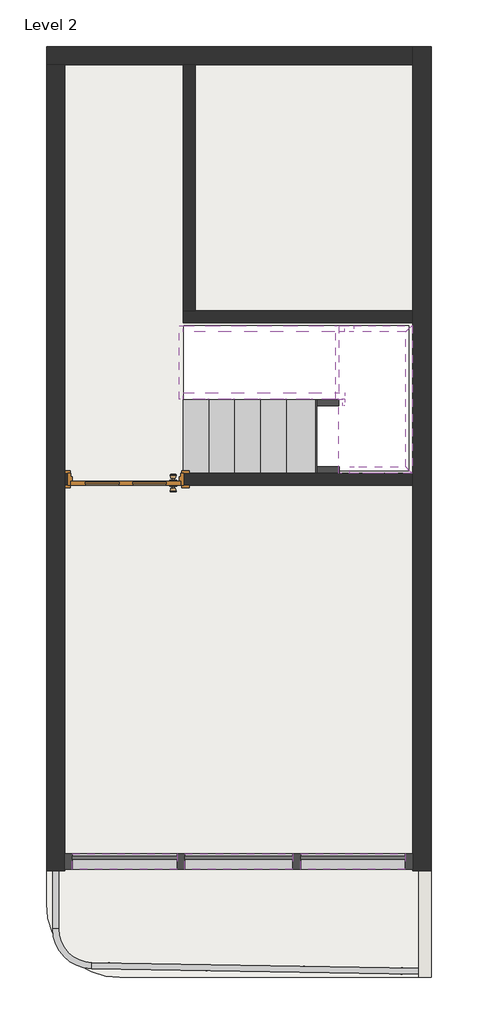
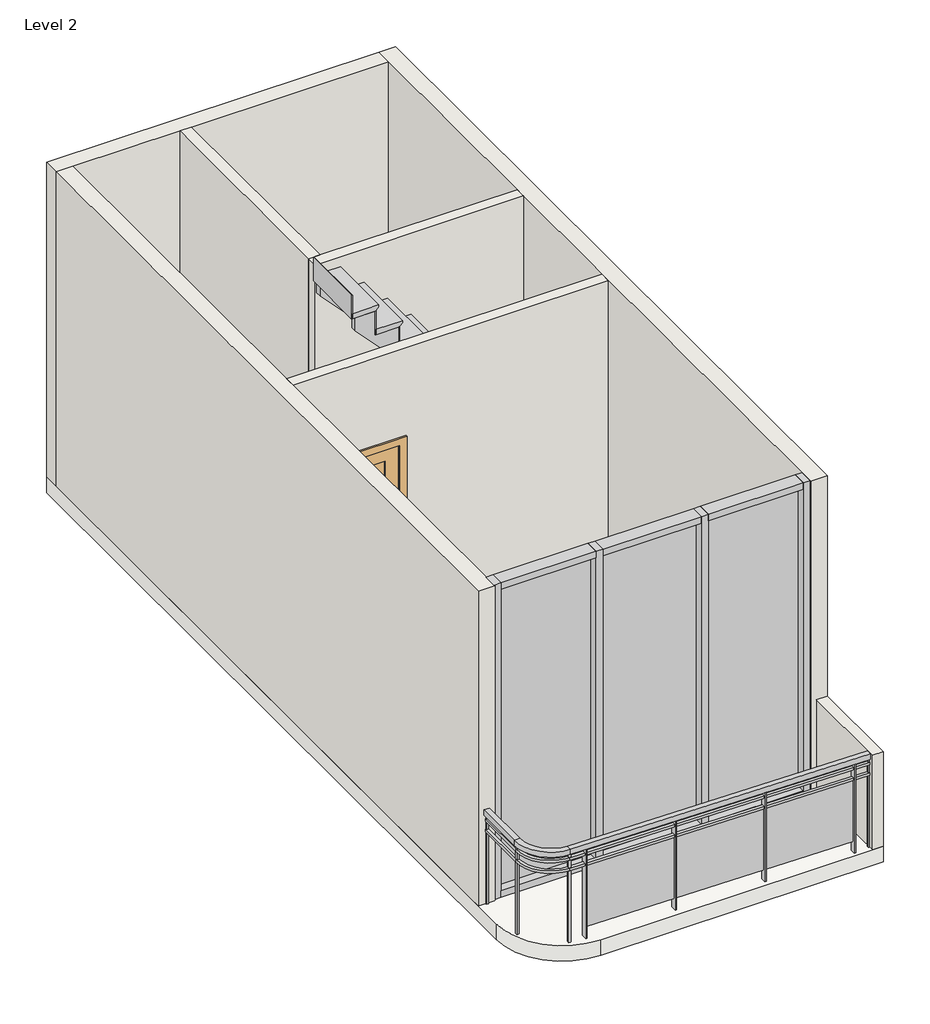
# One storey: 18 members, 7 walls, 3 plates, 2 slabs, 2 stair flights, 1 door, 1 railing.
"""IFC4 building model written with IfcOpenShell, lengths in millimetres."""

from ifc_helpers import new_model, si_unit, point, frame, frame_2d, origin, place, context, project, spatial, polyline, circle_curve, trimmed, segment, composite_curve, outline, extrude, faceted_brep, transform, mapped, element, save
from ifc_brep_helpers import plane_surface, cylinder_surface, revolved_surface, advanced_brep
from components import door_interior_single_4_panel_wood_3_aef61117, member_024c663a, member_b7368e82, member_eaba9652, member_3f395ae9, system_panel_glazed_640eda3d, system_panel_glazed_15df7e53, non_monolithic_landing_067df1a0, stair_flight_7576936b, stair_flight_48b2ccee

model = new_model("IFC4")

# Units and contexts
model_context = context("Model", 3, world=origin())
ifc_project = project(units=[si_unit("LENGTHUNIT", "METRE", prefix="MILLI")], contexts=[model_context])

# Site, building, storey
site = spatial("IfcSite", under=ifc_project)
building = spatial("IfcBuilding", under=site)
storey = spatial("IfcBuildingStorey", under=building, Name="Level 2", Elevation=3200.4)

# Door
placement = place(None, origin())
door_interior_single_4_panel_wood_3_shape = door_interior_single_4_panel_wood_3_aef61117(model_context)
element("IfcDoor", 1, ObjectType="Door-Interior-Single-4_Panel-Wood : 3'", at=placement, inside=storey, context=model_context, shape_type="MappedRepresentation", body=[
    mapped(door_interior_single_4_panel_wood_3_shape, transform((-5067.456559, 3670.9730625, 3200.4), x_axis=(-1.0, 0.0, 0.0), y_axis=(0.0, -1.0, 0.0), z_axis=(0.0, 0.0, 1.0))),
])

# Members
element("IfcMember", 2, ObjectType="Carriage - 2\" Width", at=placement, inside=storey, context=model_context, shape_type="Brep", body=[
    faceted_brep([(-3327.7737097, 4341.1083475, 4978.4), (-3327.7737097, 4391.9083475, 4978.4), (-3543.6737097, 4391.9083475, 4978.4), (-3543.6737097, 4341.1083475, 4978.4), (-3327.7737097, 4341.1083475, 4749.8), (-3327.7737097, 4391.9083475, 4749.8), (-3543.6737097, 4341.1083475, 5207.0), (-3543.6737097, 4391.9083475, 5207.0), (-3759.5737097, 4391.9083475, 5207.0), (-3759.5737097, 4341.1083475, 5207.0), (-3759.5737097, 4341.1083475, 5435.6), (-3759.5737097, 4391.9083475, 5435.6), (-3975.4737097, 4391.9083475, 5435.6), (-3975.4737097, 4341.1083475, 5435.6), (-3975.4737097, 4341.1083475, 5664.2), (-3975.4737097, 4391.9083475, 5664.2), (-4191.3737097, 4391.9083475, 5664.2), (-4191.3737097, 4341.1083475, 5664.2), (-4191.3737097, 4341.1083475, 5892.8), (-4191.3737097, 4391.9083475, 5892.8), (-4407.2737097, 4391.9083475, 5892.8), (-4407.2737097, 4341.1083475, 5892.8), (-4407.2737097, 4341.1083475, 6121.4), (-4407.2737097, 4391.9083475, 6121.4), (-4591.4237097, 4391.9083475, 6121.4), (-4591.4237097, 4341.1083475, 6121.4), (-3245.2237097, 4341.1083475, 4572.0), (-3245.2237097, 4391.9083475, 4572.0), (-3245.2237097, 4391.9083475, 4749.8), (-3245.2237097, 4341.1083475, 4749.8), (-3247.1951617, 4341.1083475, 4572.0), (-3247.1951617, 4391.9083475, 4572.0), (-4591.4237097, 4391.9083475, 5995.3008155), (-4591.4237097, 4341.1083475, 5995.3008155), (-3296.0237097, 4341.1083475, 4623.7008155), (-3327.7737097, 4341.1083475, 4657.3184625), (-3543.6737097, 4341.1083475, 4885.9184625), (-3759.5737097, 4341.1083475, 5114.5184625), (-3975.4737097, 4341.1083475, 5343.1184625), (-4191.3737097, 4341.1083475, 5571.7184625), (-4407.2737097, 4341.1083475, 5800.3184625), (-3296.0237097, 4341.1083475, 4749.8)], [[[0, 1, 2, 3]], [[1, 0, 4, 5]], [[6, 7, 8, 9]], [[3, 2, 7, 6]], [[10, 11, 12, 13]], [[9, 8, 11, 10]], [[14, 15, 16, 17]], [[13, 12, 15, 14]], [[18, 19, 20, 21]], [[17, 16, 19, 18]], [[22, 23, 24, 25]], [[21, 20, 23, 22]], [[26, 27, 28, 29]], [[26, 30, 31, 27]], [[32, 33, 25, 24]], [[31, 32, 24, 23, 20, 19, 16, 15, 12, 11, 8, 7, 2, 1, 5, 28, 27]], [[33, 32, 31, 30, 34, 35, 36, 37, 38, 39, 40]], [[30, 26, 29, 41, 4, 0, 3, 6, 9, 10, 13, 14, 17, 18, 21, 22, 25, 33, 40, 39, 38, 37, 36, 35, 34]], [[5, 4, 41, 29, 28]]]),
])
element("IfcMember", 3, ObjectType="Carriage - 2\" Width", at=placement, inside=storey, context=model_context, shape_type="Brep", body=[
    faceted_brep([(-4591.4237097, 4950.7083475, 5995.3008155), (-4591.4237097, 4899.9083475, 5995.3008155), (-4591.4237097, 4899.9083475, 6121.4), (-4591.4237097, 4950.7083475, 6121.4), (-3247.1951617, 4899.9083475, 4572.0), (-3170.555096, 4899.9083475, 4749.8), (-3327.7737097, 4899.9083475, 4749.8), (-3327.7737097, 4899.9083475, 4978.4), (-3543.6737097, 4899.9083475, 4978.4), (-3543.6737097, 4899.9083475, 5207.0), (-3759.5737097, 4899.9083475, 5207.0), (-3759.5737097, 4899.9083475, 5435.6), (-3975.4737097, 4899.9083475, 5435.6), (-3975.4737097, 4899.9083475, 5664.2), (-4191.3737097, 4899.9083475, 5664.2), (-4191.3737097, 4899.9083475, 5892.8), (-4407.2737097, 4899.9083475, 5892.8), (-4407.2737097, 4899.9083475, 6121.4), (-4407.2737097, 4950.7083475, 5800.3184625), (-4191.3737097, 4950.7083475, 5571.7184625), (-3975.4737097, 4950.7083475, 5343.1184625), (-3759.5737097, 4950.7083475, 5114.5184625), (-3543.6737097, 4950.7083475, 4885.9184625), (-3327.7737097, 4950.7083475, 4657.3184625), (-3296.0237097, 4950.7083475, 4623.7008155), (-3247.1951617, 4950.7083475, 4572.0), (-4407.2737097, 4950.7083475, 6121.4), (-4407.2737097, 4950.7083475, 5892.8), (-4191.3737097, 4950.7083475, 5892.8), (-4191.3737097, 4950.7083475, 5664.2), (-3975.4737097, 4950.7083475, 5664.2), (-3975.4737097, 4950.7083475, 5435.6), (-3759.5737097, 4950.7083475, 5435.6), (-3759.5737097, 4950.7083475, 5207.0), (-3543.6737097, 4950.7083475, 5207.0), (-3543.6737097, 4950.7083475, 4978.4), (-3327.7737097, 4950.7083475, 4978.4), (-3327.7737097, 4950.7083475, 4749.8), (-3296.0237097, 4950.7083475, 4749.8), (-3170.555096, 4950.7083475, 4749.8)], [[[0, 1, 2, 3]], [[1, 4, 5, 6, 7, 8, 9, 10, 11, 12, 13, 14, 15, 16, 17, 2]], [[1, 0, 18, 19, 20, 21, 22, 23, 24, 25, 4]], [[0, 3, 26, 27, 28, 29, 30, 31, 32, 33, 34, 35, 36, 37, 38, 39, 25, 24, 23, 22, 21, 20, 19, 18]], [[7, 36, 35, 8]], [[36, 7, 6, 37]], [[9, 34, 33, 10]], [[8, 35, 34, 9]], [[11, 32, 31, 12]], [[10, 33, 32, 11]], [[13, 30, 29, 14]], [[12, 31, 30, 13]], [[15, 28, 27, 16]], [[14, 29, 28, 15]], [[17, 26, 3, 2]], [[16, 27, 26, 17]], [[4, 25, 39, 5]], [[37, 6, 5, 39, 38]]]),
])
element("IfcMember", 4, ObjectType="Carriage - 2\" Width", at=placement, inside=storey, context=model_context, shape_type="Brep", body=[
    faceted_brep([(-4559.6737097, 4334.5480625, 3200.4), (-4424.3522576, 4334.5480625, 3200.4), (-4424.3522576, 4283.7480625, 3200.4), (-4559.6737097, 4283.7480625, 3200.4), (-3296.0237097, 4334.5480625, 4395.1008155), (-3296.0237097, 4283.7480625, 4395.1008155), (-4343.7737097, 4334.5480625, 3285.7184625), (-4127.8737097, 4334.5480625, 3514.3184625), (-3911.9737097, 4334.5480625, 3742.9184625), (-3696.0737097, 4334.5480625, 3971.5184625), (-3480.1737097, 4334.5480625, 4200.1184625), (-3296.0237097, 4334.5480625, 4521.2), (-4559.6737097, 4334.5480625, 3378.2), (-4343.7737097, 4334.5480625, 3378.2), (-4343.7737097, 4334.5480625, 3606.8), (-4127.8737097, 4334.5480625, 3606.8), (-4127.8737097, 4334.5480625, 3835.4), (-3911.9737097, 4334.5480625, 3835.4), (-3911.9737097, 4334.5480625, 4064.0), (-3696.0737097, 4334.5480625, 4064.0), (-3696.0737097, 4334.5480625, 4292.6), (-3480.1737097, 4334.5480625, 4292.6), (-3480.1737097, 4334.5480625, 4521.2), (-3480.1737097, 4283.7480625, 4521.2), (-3296.0237097, 4283.7480625, 4521.2), (-3480.1737097, 4283.7480625, 4292.6), (-3696.0737097, 4283.7480625, 4292.6), (-3696.0737097, 4283.7480625, 4064.0), (-3911.9737097, 4283.7480625, 4064.0), (-3911.9737097, 4283.7480625, 3835.4), (-4127.8737097, 4283.7480625, 3835.4), (-4127.8737097, 4283.7480625, 3606.8), (-4343.7737097, 4283.7480625, 3606.8), (-4343.7737097, 4283.7480625, 3378.2), (-4559.6737097, 4283.7480625, 3378.2)], [[[0, 1, 2, 3]], [[4, 5, 2, 1, 6, 7, 8, 9, 10]], [[11, 4, 10, 9, 8, 7, 6, 1, 0, 12, 13, 14, 15, 16, 17, 18, 19, 20, 21, 22]], [[22, 23, 24, 11]], [[2, 5, 24, 23, 25, 26, 27, 28, 29, 30, 31, 32, 33, 34, 3]], [[34, 12, 0, 3]], [[12, 34, 33, 13]], [[13, 33, 32, 14]], [[14, 32, 31, 15]], [[15, 31, 30, 16]], [[16, 30, 29, 17]], [[17, 29, 28, 18]], [[18, 28, 27, 19]], [[19, 27, 26, 20]], [[20, 26, 25, 21]], [[21, 25, 23, 22]], [[5, 4, 11, 24]]]),
])
element("IfcMember", 5, ObjectType="Carriage - 2\" Width", at=placement, inside=storey, context=model_context, shape_type="Brep", body=[
    faceted_brep([(-4559.6737097, 3775.7480625, 3200.4), (-4424.3522576, 3775.7480625, 3200.4), (-4424.3522576, 3724.9480625, 3200.4), (-4559.6737097, 3724.9480625, 3200.4), (-3128.9522576, 3775.7480625, 4572.0), (-3128.9522576, 3724.9480625, 4572.0), (-3264.2737097, 3724.9480625, 4428.7184625), (-3296.0237097, 3724.9480625, 4395.1008155), (-3480.1737097, 3724.9480625, 4200.1184625), (-3696.0737097, 3724.9480625, 3971.5184625), (-3911.9737097, 3724.9480625, 3742.9184625), (-4127.8737097, 3724.9480625, 3514.3184625), (-4343.7737097, 3724.9480625, 3285.7184625), (-3205.5923234, 3775.7480625, 4749.8), (-4559.6737097, 3775.7480625, 3378.2), (-4343.7737097, 3775.7480625, 3378.2), (-4343.7737097, 3775.7480625, 3606.8), (-4127.8737097, 3775.7480625, 3606.8), (-4127.8737097, 3775.7480625, 3835.4), (-3911.9737097, 3775.7480625, 3835.4), (-3911.9737097, 3775.7480625, 4064.0), (-3696.0737097, 3775.7480625, 4064.0), (-3696.0737097, 3775.7480625, 4292.6), (-3480.1737097, 3775.7480625, 4292.6), (-3480.1737097, 3775.7480625, 4521.2), (-3264.2737097, 3775.7480625, 4521.2), (-3264.2737097, 3775.7480625, 4749.8), (-3480.1737097, 3724.9480625, 4521.2), (-3296.0237097, 3724.9480625, 4521.2), (-3264.2737097, 3724.9480625, 4521.2), (-3205.5923234, 3724.9480625, 4749.8), (-3264.2737097, 3724.9480625, 4749.8), (-3480.1737097, 3724.9480625, 4292.6), (-3696.0737097, 3724.9480625, 4292.6), (-3696.0737097, 3724.9480625, 4064.0), (-3911.9737097, 3724.9480625, 4064.0), (-3911.9737097, 3724.9480625, 3835.4), (-4127.8737097, 3724.9480625, 3835.4), (-4127.8737097, 3724.9480625, 3606.8), (-4343.7737097, 3724.9480625, 3606.8), (-4343.7737097, 3724.9480625, 3378.2), (-4559.6737097, 3724.9480625, 3378.2)], [[[0, 1, 2, 3]], [[4, 5, 6, 7, 8, 9, 10, 11, 12, 2, 1]], [[13, 4, 1, 0, 14, 15, 16, 17, 18, 19, 20, 21, 22, 23, 24, 25, 26]], [[24, 27, 28, 29, 25]], [[5, 30, 31, 29, 28, 27, 32, 33, 34, 35, 36, 37, 38, 39, 40, 41, 3, 2, 12, 11, 10, 9, 8, 7, 6]], [[41, 14, 0, 3]], [[14, 41, 40, 15]], [[15, 40, 39, 16]], [[16, 39, 38, 17]], [[17, 38, 37, 18]], [[18, 37, 36, 19]], [[19, 36, 35, 20]], [[20, 35, 34, 21]], [[21, 34, 33, 22]], [[22, 33, 32, 23]], [[23, 32, 27, 24]], [[5, 4, 13, 30]], [[25, 29, 31, 26]], [[26, 31, 30, 13]]]),
])
element("IfcMember", 6, ObjectType="Carriage - 2\" Width", at=placement, inside=storey, context=model_context, shape_type="SweptSolid", body=[
    extrude(outline(polyline([(-3245.2237097, 4341.1083475), (-3245.2237097, 4283.7480625), (-3264.2737097, 4283.7480625), (-3264.2737097, 4334.5480625), (-3296.0237097, 4334.5480625), (-3296.0237097, 4341.1083475), (-3245.2237097, 4341.1083475)])), frame((0.0, 0.0, 4572.0), z_axis=(0.0, 0.0, 1.0), x_axis=(1.0, 0.0, 0.0)), (0.0, 0.0, 1.0), 177.8),
])
element("IfcMember", 7, ObjectType="Carriage - 2\" Width", at=placement, inside=storey, context=model_context, shape_type="Brep", body=[
    faceted_brep([(-2737.2237097, 3775.7480625, 4572.0), (-3128.9522576, 3775.7480625, 4572.0), (-3205.5923234, 3775.7480625, 4749.8), (-2737.2237097, 3775.7480625, 4749.8), (-2686.4237097, 3724.9480625, 4572.0), (-3128.9522576, 3724.9480625, 4572.0), (-2686.4237097, 3724.9480625, 4749.8), (-3205.5923234, 3724.9480625, 4749.8)], [[[0, 1, 2, 3]], [[1, 0, 4, 5]], [[5, 4, 6, 7]], [[3, 2, 7, 6]], [[1, 5, 7, 2]], [[4, 0, 3, 6]]]),
])
element("IfcMember", 8, ObjectType="Carriage - 2\" Width", at=placement, inside=storey, context=model_context, shape_type="SweptSolid", body=[
    extrude(outline(polyline([(-2737.2237097, 3775.7480625), (-2737.2237097, 4899.9083475), (-2686.4237097, 4950.7083475), (-2686.4237097, 3724.9480625), (-2737.2237097, 3775.7480625)])), frame((0.0, 0.0, 4572.0), z_axis=(0.0, 0.0, 1.0), x_axis=(1.0, 0.0, 0.0)), (0.0, 0.0, 1.0), 177.8),
])
element("IfcMember", 9, ObjectType="Carriage - 2\" Width", at=placement, inside=storey, context=model_context, shape_type="Brep", body=[
    faceted_brep([(-3247.1951617, 4899.9083475, 4572.0), (-2737.2237097, 4899.9083475, 4572.0), (-2737.2237097, 4899.9083475, 4749.8), (-3170.555096, 4899.9083475, 4749.8), (-3247.1951617, 4950.7083475, 4572.0), (-2686.4237097, 4950.7083475, 4572.0), (-3170.555096, 4950.7083475, 4749.8), (-2686.4237097, 4950.7083475, 4749.8)], [[[0, 1, 2, 3]], [[1, 0, 4, 5]], [[5, 4, 6, 7]], [[3, 2, 7, 6]], [[1, 5, 7, 2]], [[4, 0, 3, 6]]]),
])
member_shape = member_024c663a(model_context)
element("IfcMember", 10, ObjectType="Rectangular Mullion : 2.5\" x 5\" rectangular", at=placement, inside=storey, context=model_context, shape_type="MappedRepresentation", body=[
    mapped(member_shape, transform((-2743.356559, 492.7980625, 6248.4), x_axis=(0.0, 0.0, 1.0), y_axis=(0.0, -1.0, 0.0), z_axis=(1.0, 0.0, 0.0))),
])
element("IfcMember", 11, ObjectType="Rectangular Mullion : 2.5\" x 5\" rectangular", at=placement, inside=storey, context=model_context, shape_type="MappedRepresentation", body=[
    mapped(member_shape, transform((-4642.006559, 492.7980625, 6248.4), x_axis=(0.0, 0.0, 1.0), y_axis=(0.0, -1.0, 0.0), z_axis=(1.0, 0.0, 0.0))),
])
element("IfcMember", 12, ObjectType="Rectangular Mullion : 2.5\" x 5\" rectangular", at=placement, inside=storey, context=model_context, shape_type="MappedRepresentation", body=[
    mapped(member_shape, transform((-5511.956559, 492.7980625, 3200.4), x_axis=(0.0, 0.0, -1.0), y_axis=(0.0, -1.0, 0.0), z_axis=(-1.0, 0.0, 0.0))),
])
element("IfcMember", 13, ObjectType="Rectangular Mullion : 2.5\" x 5\" rectangular", at=placement, inside=storey, context=model_context, shape_type="MappedRepresentation", body=[
    mapped(member_shape, transform((-3613.306559, 492.7980625, 3200.4), x_axis=(0.0, 0.0, -1.0), y_axis=(0.0, -1.0, 0.0), z_axis=(-1.0, 0.0, 0.0))),
])
member_2_shape = member_b7368e82(model_context)
element("IfcMember", 14, ObjectType="Rectangular Mullion : 2.5\" x 5\" rectangular", at=placement, inside=storey, context=model_context, shape_type="MappedRepresentation", body=[
    mapped(member_2_shape, transform((-4578.506559, 492.7980625, 3200.4), x_axis=(0.0, 0.0, -1.0), y_axis=(0.0, -1.0, 0.0), z_axis=(-1.0, 0.0, 0.0))),
])
element("IfcMember", 15, ObjectType="Rectangular Mullion : 2.5\" x 5\" rectangular", at=placement, inside=storey, context=model_context, shape_type="MappedRepresentation", body=[
    mapped(member_2_shape, transform((-3676.806559, 492.7980625, 6248.4), x_axis=(0.0, 0.0, 1.0), y_axis=(0.0, -1.0, 0.0), z_axis=(1.0, 0.0, 0.0))),
])
member_3_shape = member_eaba9652(model_context)
element("IfcMember", 16, ObjectType="Rectangular Mullion : 2.5\" x 5\" rectangular", at=placement, inside=storey, context=model_context, shape_type="MappedRepresentation", body=[
    mapped(member_3_shape, transform((-4610.256559, 492.7980625, 3200.4), x_axis=(1.0, 0.0, 0.0), y_axis=(0.0, -1.0, 0.0), z_axis=(0.0, 0.0, -1.0))),
])
element("IfcMember", 17, ObjectType="Rectangular Mullion : 2.5\" x 5\" rectangular", at=placement, inside=storey, context=model_context, shape_type="MappedRepresentation", body=[
    mapped(member_3_shape, transform((-3645.056559, 492.7980625, 3200.4), x_axis=(1.0, 0.0, 0.0), y_axis=(0.0, -1.0, 0.0), z_axis=(0.0, 0.0, -1.0))),
])
member_4_shape = member_3f395ae9(model_context)
element("IfcMember", 18, ObjectType="Rectangular Mullion : 2.5\" x 5\" rectangular", at=placement, inside=storey, context=model_context, shape_type="MappedRepresentation", body=[
    mapped(member_4_shape, transform((-2679.856559, 492.7980625, 3200.4), x_axis=(1.0, 0.0, 0.0), y_axis=(0.0, -1.0, 0.0), z_axis=(0.0, 0.0, -1.0))),
])
element("IfcMember", 19, ObjectType="Rectangular Mullion : 2.5\" x 5\" rectangular", at=placement, inside=storey, context=model_context, shape_type="MappedRepresentation", body=[
    mapped(member_4_shape, transform((-5575.456559, 492.7980625, 6248.4), x_axis=(-1.0, 0.0, 0.0), y_axis=(0.0, -1.0, 0.0), z_axis=(0.0, 0.0, 1.0))),
])

# Plates
system_panel_glazed_shape = system_panel_glazed_640eda3d(model_context)
element("IfcPlate", 20, ObjectType="System Panel : Glazed", at=placement, inside=storey, context=model_context, shape_type="MappedRepresentation", body=[
    mapped(system_panel_glazed_shape, transform((-5076.981559, 492.7980625, 3263.9), x_axis=(1.0, 0.0, 0.0), y_axis=(0.0, 1.0, 0.0), z_axis=(0.0, 0.0, 1.0))),
])
element("IfcPlate", 21, ObjectType="System Panel : Glazed", at=placement, inside=storey, context=model_context, shape_type="MappedRepresentation", body=[
    mapped(system_panel_glazed_shape, transform((-3178.331559, 492.7980625, 3263.9), x_axis=(1.0, 0.0, 0.0), y_axis=(0.0, 1.0, 0.0), z_axis=(0.0, 0.0, 1.0))),
])
system_panel_glazed_2_shape = system_panel_glazed_15df7e53(model_context)
element("IfcPlate", 22, ObjectType="System Panel : Glazed", at=placement, inside=storey, context=model_context, shape_type="MappedRepresentation", body=[
    mapped(system_panel_glazed_2_shape, transform((-4127.656559, 492.7980625, 3263.9), x_axis=(1.0, 0.0, 0.0), y_axis=(0.0, 1.0, 0.0), z_axis=(0.0, 0.0, 1.0))),
])

# Railing
element("IfcRailing", 23, ObjectType="Glass Panel - Bottom Fill", at=placement, inside=storey, context=model_context, shape_type="SolidModel", body=[
    advanced_brep(
    [(-2629.4642329, -446.998069, 4114.8), (-2629.4642329, -446.998069, 4064.0), (-2628.5776506, -396.2058061, 4064.0), (-2628.5776506, -396.2058061, 4114.8), (-5352.6193436, -399.4652197, 4114.8), (-5352.6193436, -399.4652197, 4064.0), (-5351.7327614, -348.6729568, 4064.0), (-5351.7327614, -348.6729568, 4114.8), (-5677.056559, -69.3155108, 4064.0), (-5677.056559, -69.3155108, 4114.8), (-5626.256559, -69.3155108, 4064.0), (-5626.256559, -69.3155108, 4114.8), (-5677.056559, 416.5980625, 4114.8), (-5626.256559, 416.5980625, 4114.8), (-5626.256559, 416.5980625, 4064.0), (-5677.056559, 416.5980625, 4064.0)],
    [
        (0, 1),
        (1, 2),
        (2, 3),
        (3, 0),
        (0, 4),
        (4, 5),
        (5, 1),
        (5, 6),
        (6, 2),
        (6, 7),
        (7, 3),
        (7, 4),
        (8, 5, circle_curve(frame((-5346.856559, -69.3155108, 4064.0), z_axis=(0.0, 0.0, 1.0), x_axis=(-0.017452406437286138, -0.9998476951563912, 0.0)), 330.2)),
        (4, 9, circle_curve(frame((-5346.856559, -69.3155108, 4114.8), z_axis=(0.0, 0.0, -1.0), x_axis=(-0.017452406437286138, -0.9998476951563912, 0.0)), 330.2)),
        (9, 8),
        (10, 6, circle_curve(frame((-5346.856559, -69.3155108, 4064.0), z_axis=(0.0, 0.0, 1.0), x_axis=(-0.017452406437286138, -0.9998476951563912, 0.0)), 279.4)),
        (8, 10),
        (11, 7, circle_curve(frame((-5346.856559, -69.3155108, 4114.8), z_axis=(0.0, 0.0, 1.0), x_axis=(-0.017452406437286138, -0.9998476951563912, 0.0)), 279.4)),
        (10, 11),
        (11, 9),
        (12, 13),
        (13, 14),
        (14, 15),
        (15, 12),
        (9, 12),
        (15, 8),
        (14, 10),
        (13, 11),
    ],
    [
        plane_surface(frame((-2629.0209418, -421.6019375, 4114.8), z_axis=(0.9998476951563912, -0.017452406437286544, 0.0), x_axis=(0.017452406437286544, 0.9998476951563912, 0.0))),
        plane_surface(frame((-2629.4642329, -446.998069, 4114.8), z_axis=(-0.017452406437286554, -0.9998476951563912, 0.0), x_axis=(-0.9998476951563912, 0.017452406437286554, 0.0))),
        plane_surface(frame((-2629.4642329, -446.998069, 4064.0), z_axis=(0.0, 0.0, -1.0), x_axis=(-0.9998476951563912, 0.017452406437286554, 0.0))),
        plane_surface(frame((-2628.5776506, -396.2058061, 4064.0), z_axis=(0.017452406437286547, 0.9998476951563912, 0.0), x_axis=(-0.9998476951563912, 0.017452406437286547, 0.0))),
        plane_surface(frame((-2628.5776506, -396.2058061, 4114.8), z_axis=(0.0, 0.0, 1.0), x_axis=(-0.9998476951563912, 0.017452406437286547, 0.0))),
        cylinder_surface(frame((-5346.856559, -69.3155108, 4114.8), z_axis=(0.0, 0.0, -1.0), x_axis=(-0.017452406437286138, -0.9998476951563912, 0.0)), 330.2),
        plane_surface(frame((-5346.856559, -69.3155108, 4064.0), z_axis=(0.0, 0.0, -1.0000000000000002), x_axis=(-0.01745240643728614, -0.9998476951563913, 0.0))),
        revolved_surface(polyline([(-5351.732761358578, -348.67295682669567, 4064.0), (-5351.732761358578, -348.67295682669567, 4114.8)]), (-5346.856559, -69.3155108, 4114.8), (0.0, 0.0, -1.0)),
        plane_surface(frame((-5346.856559, -69.3155108, 4114.8), z_axis=(0.0, 0.0, 1.0000000000000002), x_axis=(-0.01745240643728614, -0.9998476951563913, 0.0))),
        plane_surface(frame((-5651.656559, 416.5980625, 4114.8), z_axis=(0.0, 1.0, 0.0), x_axis=(0.0, 0.0, 1.0))),
        plane_surface(frame((-5677.056559, -69.3155108, 4114.8), z_axis=(-1.0, 0.0, 0.0), x_axis=(0.0, 1.0, 0.0))),
        plane_surface(frame((-5677.056559, -69.3155108, 4064.0), z_axis=(0.0, 0.0, -1.0), x_axis=(0.0, 1.0, 0.0))),
        plane_surface(frame((-5626.256559, -69.3155108, 4064.0), z_axis=(1.0, 0.0, 0.0), x_axis=(0.0, 1.0, 0.0))),
        plane_surface(frame((-5626.256559, -69.3155108, 4114.8), z_axis=(0.0, 0.0, 1.0), x_axis=(0.0, 1.0, 0.0))),
    ],
    [
        (0, [[1, 2, 3, 4]]),
        (1, [[-1, 5, 6, 7]]),
        (2, [[-2, -7, 8, 9]]),
        (3, [[-3, -9, 10, 11]]),
        (4, [[-4, -11, 12, -5]]),
        (5, [[13, -6, 14, 15]]),
        (6, [[16, -8, -13, 17]]),
        (7, [[18, -10, -16, 19]]),
        (8, [[-14, -12, -18, 20]]),
        (9, [[21, 22, 23, 24]]),
        (10, [[-15, 25, -24, 26]]),
        (11, [[-17, -26, -23, 27]]),
        (12, [[-19, -27, -22, 28]]),
        (13, [[-20, -28, -21, -25]]),
    ],
),
    advanced_brep(
    [(-2628.7992962, -408.9038718, 4025.9), (-2629.2425873, -434.3000032, 4025.9), (-2629.2425873, -434.3000032, 4000.5), (-2628.7992962, -408.9038718, 4000.5), (-5351.9544069, -361.3710225, 4025.9), (-5352.3976981, -386.767154, 4025.9), (-5352.3976981, -386.767154, 4000.5), (-5351.9544069, -361.3710225, 4000.5), (-5664.356559, -69.3155108, 4025.9), (-5638.956559, -69.3155108, 4025.9), (-5664.356559, -69.3155108, 4000.5), (-5638.956559, -69.3155108, 4000.5), (-5638.956559, 416.5980625, 4025.9), (-5638.956559, 416.5980625, 4000.5), (-5664.356559, 416.5980625, 4000.5), (-5664.356559, 416.5980625, 4025.9)],
    [
        (0, 1),
        (1, 2),
        (2, 3),
        (3, 0),
        (0, 4),
        (4, 5),
        (5, 1),
        (5, 6),
        (6, 2),
        (6, 7),
        (7, 3),
        (7, 4),
        (8, 5, circle_curve(frame((-5346.856559, -69.3155108, 4025.9), z_axis=(0.0, 0.0, 1.0), x_axis=(-0.017452406437286138, -0.9998476951563912, 0.0)), 317.5)),
        (4, 9, circle_curve(frame((-5346.856559, -69.3155108, 4025.9), z_axis=(0.0, 0.0, -1.0), x_axis=(-0.017452406437286138, -0.9998476951563912, 0.0)), 292.1)),
        (9, 8),
        (10, 6, circle_curve(frame((-5346.856559, -69.3155108, 4000.5), z_axis=(0.0, 0.0, 1.0), x_axis=(-0.017452406437286138, -0.9998476951563912, 0.0)), 317.5)),
        (8, 10),
        (11, 7, circle_curve(frame((-5346.856559, -69.3155108, 4000.5), z_axis=(0.0, 0.0, 1.0), x_axis=(-0.017452406437286138, -0.9998476951563912, 0.0)), 292.1)),
        (10, 11),
        (11, 9),
        (12, 13),
        (13, 14),
        (14, 15),
        (15, 12),
        (9, 12),
        (15, 8),
        (14, 10),
        (13, 11),
    ],
    [
        plane_surface(frame((-2629.0209418, -421.6019375, 4013.2), z_axis=(0.9998476951563912, -0.017452406437286544, 0.0), x_axis=(0.017452406437286544, 0.9998476951563912, 0.0))),
        plane_surface(frame((-2628.7992962, -408.9038718, 4025.9), z_axis=(0.0, 0.0, 1.0), x_axis=(-0.9998476951563912, 0.017452406437286554, 0.0))),
        plane_surface(frame((-2629.2425873, -434.3000032, 4025.9), z_axis=(-0.017452406437286547, -0.9998476951563912, 0.0), x_axis=(-0.9998476951563912, 0.017452406437286547, 0.0))),
        plane_surface(frame((-2629.2425873, -434.3000032, 4000.5), z_axis=(0.0, 0.0, -1.0), x_axis=(-0.9998476951563912, 0.017452406437286547, 0.0))),
        plane_surface(frame((-2628.7992962, -408.9038718, 4000.5), z_axis=(0.017452406437286554, 0.9998476951563912, 0.0), x_axis=(-0.9998476951563912, 0.017452406437286554, 0.0))),
        plane_surface(frame((-5346.856559, -69.3155108, 4025.9), z_axis=(0.0, 0.0, 1.0000000000000002), x_axis=(-0.01745240643728614, -0.9998476951563913, 0.0))),
        cylinder_surface(frame((-5346.856559, -69.3155108, 4013.2), z_axis=(0.0, 0.0, -1.0), x_axis=(-0.017452406437286138, -0.9998476951563912, 0.0)), 317.5),
        plane_surface(frame((-5346.856559, -69.3155108, 4000.5), z_axis=(0.0, 0.0, -1.0000000000000002), x_axis=(-0.01745240643728614, -0.9998476951563913, 0.0))),
        revolved_surface(polyline([(-5351.954406920331, -361.37102255518187, 4000.5), (-5351.954406920331, -361.37102255518187, 4025.9)]), (-5346.856559, -69.3155108, 4013.2), (0.0, 0.0, -1.0)),
        plane_surface(frame((-5651.656559, 416.5980625, 4013.2), z_axis=(0.0, 1.0, 0.0), x_axis=(0.0, 0.0, 1.0))),
        plane_surface(frame((-5638.956559, -69.3155108, 4025.9), z_axis=(0.0, 0.0, 1.0), x_axis=(0.0, 1.0, 0.0))),
        plane_surface(frame((-5664.356559, -69.3155108, 4025.9), z_axis=(-1.0, 0.0, 0.0), x_axis=(0.0, 1.0, 0.0))),
        plane_surface(frame((-5664.356559, -69.3155108, 4000.5), z_axis=(0.0, 0.0, -1.0), x_axis=(0.0, 1.0, 0.0))),
        plane_surface(frame((-5638.956559, -69.3155108, 4000.5), z_axis=(1.0, 0.0, 0.0), x_axis=(0.0, 1.0, 0.0))),
    ],
    [
        (0, [[1, 2, 3, 4]]),
        (1, [[-1, 5, 6, 7]]),
        (2, [[-2, -7, 8, 9]]),
        (3, [[-3, -9, 10, 11]]),
        (4, [[-4, -11, 12, -5]]),
        (5, [[13, -6, 14, 15]]),
        (6, [[16, -8, -13, 17]]),
        (7, [[18, -10, -16, 19]]),
        (8, [[-14, -12, -18, 20]]),
        (9, [[21, 22, 23, 24]]),
        (10, [[-15, 25, -24, 26]]),
        (11, [[-17, -26, -23, 27]]),
        (12, [[-19, -27, -22, 28]]),
        (13, [[-20, -28, -21, -25]]),
    ],
),
    advanced_brep(
    [(-2628.7992962, -408.9038718, 3924.3), (-2629.2425873, -434.3000032, 3924.3), (-2629.2425873, -434.3000032, 3898.9), (-2628.7992962, -408.9038718, 3898.9), (-5351.9544069, -361.3710225, 3924.3), (-5352.3976981, -386.767154, 3924.3), (-5352.3976981, -386.767154, 3898.9), (-5351.9544069, -361.3710225, 3898.9), (-5664.356559, -69.3155108, 3924.3), (-5638.956559, -69.3155108, 3924.3), (-5664.356559, -69.3155108, 3898.9), (-5638.956559, -69.3155108, 3898.9), (-5638.956559, 416.5980625, 3924.3), (-5638.956559, 416.5980625, 3898.9), (-5664.356559, 416.5980625, 3898.9), (-5664.356559, 416.5980625, 3924.3)],
    [
        (0, 1),
        (1, 2),
        (2, 3),
        (3, 0),
        (0, 4),
        (4, 5),
        (5, 1),
        (5, 6),
        (6, 2),
        (6, 7),
        (7, 3),
        (7, 4),
        (8, 5, circle_curve(frame((-5346.856559, -69.3155108, 3924.3), z_axis=(0.0, 0.0, 1.0), x_axis=(-0.017452406437286138, -0.9998476951563912, 0.0)), 317.5)),
        (4, 9, circle_curve(frame((-5346.856559, -69.3155108, 3924.3), z_axis=(0.0, 0.0, -1.0), x_axis=(-0.017452406437286138, -0.9998476951563912, 0.0)), 292.1)),
        (9, 8),
        (10, 6, circle_curve(frame((-5346.856559, -69.3155108, 3898.9), z_axis=(0.0, 0.0, 1.0), x_axis=(-0.017452406437286138, -0.9998476951563912, 0.0)), 317.5)),
        (8, 10),
        (11, 7, circle_curve(frame((-5346.856559, -69.3155108, 3898.9), z_axis=(0.0, 0.0, 1.0), x_axis=(-0.017452406437286138, -0.9998476951563912, 0.0)), 292.1)),
        (10, 11),
        (11, 9),
        (12, 13),
        (13, 14),
        (14, 15),
        (15, 12),
        (9, 12),
        (15, 8),
        (14, 10),
        (13, 11),
    ],
    [
        plane_surface(frame((-2629.0209418, -421.6019375, 3911.6), z_axis=(0.9998476951563912, -0.017452406437286544, 0.0), x_axis=(0.017452406437286544, 0.9998476951563912, 0.0))),
        plane_surface(frame((-2628.7992962, -408.9038718, 3924.3), z_axis=(0.0, 0.0, 1.0), x_axis=(-0.9998476951563912, 0.017452406437286554, 0.0))),
        plane_surface(frame((-2629.2425873, -434.3000032, 3924.3), z_axis=(-0.017452406437286547, -0.9998476951563912, 0.0), x_axis=(-0.9998476951563912, 0.017452406437286547, 0.0))),
        plane_surface(frame((-2629.2425873, -434.3000032, 3898.9), z_axis=(0.0, 0.0, -1.0), x_axis=(-0.9998476951563912, 0.017452406437286547, 0.0))),
        plane_surface(frame((-2628.7992962, -408.9038718, 3898.9), z_axis=(0.017452406437286554, 0.9998476951563912, 0.0), x_axis=(-0.9998476951563912, 0.017452406437286554, 0.0))),
        plane_surface(frame((-5346.856559, -69.3155108, 3924.3), z_axis=(0.0, 0.0, 1.0000000000000002), x_axis=(-0.01745240643728614, -0.9998476951563913, 0.0))),
        cylinder_surface(frame((-5346.856559, -69.3155108, 3911.6), z_axis=(0.0, 0.0, -1.0), x_axis=(-0.017452406437286138, -0.9998476951563912, 0.0)), 317.5),
        plane_surface(frame((-5346.856559, -69.3155108, 3898.9), z_axis=(0.0, 0.0, -1.0000000000000002), x_axis=(-0.01745240643728614, -0.9998476951563913, 0.0))),
        revolved_surface(polyline([(-5351.954406920331, -361.37102255518187, 3898.9), (-5351.954406920331, -361.37102255518187, 3924.3)]), (-5346.856559, -69.3155108, 3911.6), (0.0, 0.0, -1.0)),
        plane_surface(frame((-5651.656559, 416.5980625, 3911.6), z_axis=(0.0, 1.0, 0.0), x_axis=(0.0, 0.0, 1.0))),
        plane_surface(frame((-5638.956559, -69.3155108, 3924.3), z_axis=(0.0, 0.0, 1.0), x_axis=(0.0, 1.0, 0.0))),
        plane_surface(frame((-5664.356559, -69.3155108, 3924.3), z_axis=(-1.0, 0.0, 0.0), x_axis=(0.0, 1.0, 0.0))),
        plane_surface(frame((-5664.356559, -69.3155108, 3898.9), z_axis=(0.0, 0.0, -1.0), x_axis=(0.0, 1.0, 0.0))),
        plane_surface(frame((-5638.956559, -69.3155108, 3898.9), z_axis=(1.0, 0.0, 0.0), x_axis=(0.0, 1.0, 0.0))),
    ],
    [
        (0, [[1, 2, 3, 4]]),
        (1, [[-1, 5, 6, 7]]),
        (2, [[-2, -7, 8, 9]]),
        (3, [[-3, -9, 10, 11]]),
        (4, [[-4, -11, 12, -5]]),
        (5, [[13, -6, 14, 15]]),
        (6, [[16, -8, -13, 17]]),
        (7, [[18, -10, -16, 19]]),
        (8, [[-14, -12, -18, 20]]),
        (9, [[21, 22, 23, 24]]),
        (10, [[-15, 25, -24, 26]]),
        (11, [[-17, -26, -23, 27]]),
        (12, [[-19, -27, -22, 28]]),
        (13, [[-20, -28, -21, -25]]),
    ],
),
    extrude(outline(polyline([(-5202.8204831, -351.2722303), (-5203.7070653, -402.0644932), (-5216.4051311, -401.8428476), (-5215.5185488, -351.0505847), (-5202.8204831, -351.2722303)])), frame((0.0, 0.0, 3200.4), z_axis=(0.0, 0.0, 1.0), x_axis=(1.0, 0.0, 0.0)), (0.0, 0.0, 1.0), 863.6),
    extrude(outline(polyline([(-4397.0506547, -397.2770166), (-5209.7268613, -383.0917006), (-5209.6160385, -376.7426678), (-4396.9398319, -390.9279837), (-4397.0506547, -397.2770166)])), frame((0.0, 0.0, 3302.0), z_axis=(0.0, 0.0, 1.0), x_axis=(1.0, 0.0, 0.0)), (0.0, 0.0, 1.0), 596.9),
    extrude(outline(polyline([(-4390.1442765, -365.4575462), (-4391.0308587, -416.2498091), (-4403.7289244, -416.0281636), (-4402.8423422, -365.2359007), (-4390.1442765, -365.4575462)])), frame((0.0, 0.0, 3200.4), z_axis=(0.0, 0.0, 1.0), x_axis=(1.0, 0.0, 0.0)), (0.0, 0.0, 1.0), 863.6),
    extrude(outline(polyline([(-3584.374448, -411.4623325), (-4397.0506547, -397.2770166), (-4396.9398319, -390.9279837), (-3584.2636253, -405.1132997), (-3584.374448, -411.4623325)])), frame((0.0, 0.0, 3302.0), z_axis=(0.0, 0.0, 1.0), x_axis=(1.0, 0.0, 0.0)), (0.0, 0.0, 1.0), 596.9),
    extrude(outline(polyline([(-3577.4680698, -379.6428622), (-3578.3546521, -430.4351251), (-3591.0527178, -430.2134795), (-3590.1661356, -379.4212166), (-3577.4680698, -379.6428622)])), frame((0.0, 0.0, 3200.4), z_axis=(0.0, 0.0, 1.0), x_axis=(1.0, 0.0, 0.0)), (0.0, 0.0, 1.0), 863.6),
    extrude(outline(polyline([(-2771.6982414, -425.6476485), (-3584.374448, -411.4623325), (-3584.2636253, -405.1132997), (-2771.5874186, -419.2986156), (-2771.6982414, -425.6476485)])), frame((0.0, 0.0, 3302.0), z_axis=(0.0, 0.0, 1.0), x_axis=(1.0, 0.0, 0.0)), (0.0, 0.0, 1.0), 596.9),
    extrude(outline(polyline([(-2764.7918632, -393.8281781), (-2765.6784455, -444.6204411), (-2778.3765112, -444.3987955), (-2777.4899289, -393.6065326), (-2764.7918632, -393.8281781)])), frame((0.0, 0.0, 3200.4), z_axis=(0.0, 0.0, 1.0), x_axis=(1.0, 0.0, 0.0)), (0.0, 0.0, 1.0), 863.6),
    extrude(outline(polyline([(-5642.131559, -78.8405108), (-5661.181559, -78.8405108), (-5661.181559, -59.7905108), (-5642.131559, -59.7905108), (-5642.131559, -78.8405108)])), frame((0.0, 0.0, 3200.4), z_axis=(0.0, 0.0, 1.0), x_axis=(1.0, 0.0, 0.0)), (0.0, 0.0, 1.0), 863.6),
    extrude(outline(polyline([(-5342.486269, -364.7117731), (-5342.8187374, -383.7588717), (-5361.865836, -383.4264034), (-5361.5333676, -364.3793048), (-5342.486269, -364.7117731)])), frame((0.0, 0.0, 3200.4), z_axis=(0.0, 0.0, 1.0), x_axis=(1.0, 0.0, 0.0)), (0.0, 0.0, 1.0), 863.6),
    extrude(outline(polyline([(-5642.131559, 403.8980625), (-5661.181559, 403.8980625), (-5661.181559, 422.9480625), (-5642.131559, 422.9480625), (-5642.131559, 403.8980625)])), frame((0.0, 0.0, 3200.4), z_axis=(0.0, 0.0, 1.0), x_axis=(1.0, 0.0, 0.0)), (0.0, 0.0, 1.0), 863.6),
    extrude(outline(polyline([(-2622.5056747, -412.189211), (-2622.8381431, -431.2363096), (-2641.8852417, -430.9038413), (-2641.5527733, -411.8567427), (-2622.5056747, -412.189211)])), frame((0.0, 0.0, 3200.4), z_axis=(0.0, 0.0, 1.0), x_axis=(1.0, 0.0, 0.0)), (0.0, 0.0, 1.0), 863.6),
])

# Slabs
element("IfcSlab", 24, ObjectType="6\"", at=placement, inside=storey, context=model_context, shape_type="SweptSolid", body=[
    extrude(outline(composite_curve([segment(polyline([(-2527.456559, 7274.5980625), (-2527.456559, -472.4019375), (-5118.256559, -472.4019375)]), True, "CONTINUOUS"), segment(trimmed(circle_curve(frame_2d((-5118.256559, 137.1980625)), 609.6), [point((-5118.256559, -472.4019375))], [point((-5727.856559, 137.1980625))], False, "CARTESIAN"), True, "CONTINUOUS"), segment(polyline([(-5727.856559, 137.1980625), (-5727.856559, 7274.5980625), (-2527.456559, 7274.5980625)]), True, "CONTINUOUS")], self_intersect=False), holes=[polyline([(-4584.856559, 4950.7083475), (-4584.856559, 3743.9980625), (-2711.8237097, 3743.9980625), (-2711.8237097, 4950.7083475), (-4584.856559, 4950.7083475)])]), frame((0.0, 0.0, 3048.0), z_axis=(0.0, 0.0, 1.0), x_axis=(1.0, 0.0, 0.0)), (0.0, 0.0, 1.0), 152.4),
])
non_monolithic_landing_shape = non_monolithic_landing_067df1a0(model_context)
element("IfcSlab", 25, ObjectType="Non-Monolithic Landing", at=placement, inside=storey, context=model_context, shape_type="MappedRepresentation", body=[
    mapped(non_monolithic_landing_shape, transform((0.0, 0.0, 0.0), x_axis=(1.0, 0.0, 0.0), y_axis=(0.0, 1.0, 0.0), z_axis=(0.0, 0.0, 1.0))),
])

# Stair flights
stair_flight_shape = stair_flight_7576936b(model_context)
element("IfcStairFlight", 26, ObjectType="2\" Tread 1\" Nosing 1/4\" Riser", at=placement, inside=storey, context=model_context, shape_type="MappedRepresentation", body=[
    mapped(stair_flight_shape, transform((0.0, 0.0, 0.0), x_axis=(1.0, 0.0, 0.0), y_axis=(0.0, 1.0, 0.0), z_axis=(0.0, 0.0, 1.0))),
])
stair_flight_2_shape = stair_flight_48b2ccee(model_context)
element("IfcStairFlight", 27, ObjectType="2\" Tread 1\" Nosing 1/4\" Riser", at=placement, inside=storey, context=model_context, shape_type="MappedRepresentation", body=[
    mapped(stair_flight_2_shape, transform((0.0, 0.0, 0.0), x_axis=(1.0, 0.0, 0.0), y_axis=(0.0, 1.0, 0.0), z_axis=(0.0, 0.0, 1.0))),
])

# Walls
element("IfcWall", 28, ObjectType="4\"", at=placement, inside=storey, context=model_context, shape_type="Brep", body=[
    faceted_brep([(-2679.856559, 5077.7083475, 3200.4), (-4489.8237097, 5077.7083475, 3200.4), (-4591.4237097, 5077.7083475, 3200.4), (-4591.4237097, 5077.7083475, 6248.4), (-4489.8237097, 5077.7083475, 6248.4), (-2679.856559, 5077.7083475, 6248.4), (-2679.856559, 4976.1083475, 3200.4), (-2679.856559, 4976.1083475, 6248.4), (-4591.4237097, 4976.1083475, 6248.4), (-4591.4237097, 4976.1083475, 3200.4)], [[[0, 1, 2, 3, 4, 5]], [[6, 7, 8, 9]], [[2, 1, 0, 6, 9]], [[5, 4, 3, 8, 7]], [[0, 5, 7, 6]], [[3, 2, 9, 8]]]),
])
element("IfcWall", 29, ObjectType="4\"", at=placement, inside=storey, context=model_context, shape_type="SweptSolid", body=[
    extrude(outline(polyline([(-4489.8237097, 7122.1980625), (-4489.8237097, 5077.7083475), (-4591.4237097, 5077.7083475), (-4591.4237097, 7122.1980625), (-4489.8237097, 7122.1980625)])), frame((0.0, 0.0, 3200.4), z_axis=(0.0, 0.0, 1.0), x_axis=(1.0, 0.0, 0.0)), (0.0, 0.0, 1.0), 3048.0),
])
element("IfcWall", 30, ObjectType="4\"", at=placement, inside=storey, context=model_context, shape_type="SweptSolid", body=[
    extrude(outline(polyline([(6248.4, -2686.4237097), (6248.4, -5575.456559), (3200.4, -5575.456559), (3200.4, -5550.056559), (5359.4, -5550.056559), (5359.4, -4584.856559), (3200.4, -4584.856559), (3200.4, -2686.4237097), (6248.4, -2686.4237097)])), frame((0.0, 3623.3480625, 0.0), z_axis=(0.0, 1.0, 0.0), x_axis=(0.0, 0.0, 1.0)), (0.0, 0.0, 1.0), 101.6),
])
element("IfcWall", 31, ObjectType="4\"", at=placement, inside=storey, context=model_context, shape_type="SweptSolid", body=[
    extrude(outline(polyline([(-2629.0209418, -472.4019375), (-2629.0209418, 416.5980625), (-2527.4209418, 416.5980625), (-2527.4209418, -472.4019375), (-2629.0209418, -472.4019375)])), frame((0.0, 0.0, 3200.4), z_axis=(0.0, 0.0, 1.0), x_axis=(1.0, 0.0, 0.0)), (0.0, 0.0, 1.0), 914.4),
])
element("IfcWall", 32, ObjectType="6\"", at=placement, inside=storey, context=model_context, shape_type="Brep", body=[
    faceted_brep([(-5727.856559, 7122.1980625, 3200.4), (-5575.456559, 7122.1980625, 3200.4), (-4591.4237097, 7122.1980625, 3200.4), (-4489.8237097, 7122.1980625, 3200.4), (-2679.856559, 7122.1980625, 3200.4), (-2679.856559, 7122.1980625, 6248.4), (-4489.8237097, 7122.1980625, 6248.4), (-4591.4237097, 7122.1980625, 6248.4), (-5575.456559, 7122.1980625, 6248.4), (-5727.856559, 7122.1980625, 6248.4), (-5727.856559, 7274.5980625, 3200.4), (-5727.856559, 7274.5980625, 6248.4), (-2679.856559, 7274.5980625, 6248.4), (-2679.856559, 7274.5980625, 3200.4)], [[[0, 1, 2, 3, 4, 5, 6, 7, 8, 9]], [[10, 11, 12, 13]], [[4, 3, 2, 1, 0, 10, 13]], [[9, 8, 7, 6, 5, 12, 11]], [[0, 9, 11, 10]], [[5, 4, 13, 12]]]),
])
element("IfcWall", 33, ObjectType="6\"", at=placement, inside=storey, context=model_context, shape_type="Brep", body=[
    faceted_brep([(-2679.856559, 7274.5980625, 3200.4), (-2679.856559, 7122.1980625, 3200.4), (-2679.856559, 5077.7083475, 3200.4), (-2679.856559, 4976.1083475, 3200.4), (-2679.856559, 416.5980625, 3200.4), (-2679.856559, 416.5980625, 6248.4), (-2679.856559, 4976.1083475, 6248.4), (-2679.856559, 5077.7083475, 6248.4), (-2679.856559, 7122.1980625, 6248.4), (-2679.856559, 7274.5980625, 6248.4), (-2527.456559, 7274.5980625, 3200.4), (-2527.456559, 7274.5980625, 6248.4), (-2527.456559, 416.5980625, 6248.4), (-2527.456559, 416.5980625, 4114.8), (-2527.456559, 416.5980625, 3200.4), (-2629.0209418, 416.5980625, 3200.4)], [[[0, 1, 2, 3, 4, 5, 6, 7, 8, 9]], [[10, 11, 12, 13, 14]], [[4, 3, 2, 1, 0, 10, 14, 15]], [[5, 4, 15, 14, 13, 12]], [[9, 8, 7, 6, 5, 12, 11]], [[0, 9, 11, 10]]]),
])
element("IfcWall", 34, ObjectType="6\"", at=placement, inside=storey, context=model_context, shape_type="Brep", body=[
    faceted_brep([(-5575.456559, 416.5980625, 3200.4), (-5575.456559, 3623.3480625, 3200.4), (-5575.456559, 3724.9480625, 3200.4), (-5575.456559, 7122.1980625, 3200.4), (-5575.456559, 7122.1980625, 6248.4), (-5575.456559, 3724.9480625, 6248.4), (-5575.456559, 3623.3480625, 6248.4), (-5575.456559, 416.5980625, 6248.4), (-5727.856559, 416.5980625, 3200.4), (-5727.856559, 416.5980625, 6248.4), (-5727.856559, 7122.1980625, 6248.4), (-5727.856559, 7122.1980625, 3200.4)], [[[0, 1, 2, 3, 4, 5, 6, 7]], [[8, 9, 10, 11]], [[3, 2, 1, 0, 8, 11]], [[7, 6, 5, 4, 10, 9]], [[0, 7, 9, 8]], [[4, 3, 11, 10]]]),
])

save(model, "model.ifc")

# Revit data of these elements
# Type "Door-Interior-Single-4_Panel-Wood : 3'"
#   Type Mark = "11"
#   Assembly Code = "C1020300"
#   Analytic Construction = "Wooden"
#   Top Rail = 0' - 4 11/16"
#   Thickness = 0' - 1 3/8"
#   Thermal Resistance (R) = 2.5876 (h·ft²·°F)/BTU
#   Swing Angle [instance default] = 90.00°
#   Stiles = 0' - 4 3/4"
#   Rough Width = 3' - 2"
#   Rough Height = 7' - 1"
#   Mullion = 0' - 4 1/2"
#   Lock Rail = 0' - 7 1/2"
#   Height = 7' - 0"
#   Width = 3' - 0"
#   Heat Transfer Coefficient (U) = 0.3865 BTU/(h·ft²·°F)
#   Bottom Rail = 0' - 9 1/8"
#   Trim Material = Cherry
#   Panel Material = Cherry
#   Frame Material = Cherry
#   Door Handle Material = Aluminum
#   Visual Light Transmittance = 0
#   Solar Heat Gain Coefficient = 0
#   Wall Closure = (empty or 0)
#   Function = (empty or 0)
# Type "Rectangular Mullion : 2.5\" x 5\" rectangular"
#   built-in parameter 1007304 = 0.416667 (stored number, unit not read)
#   built-in parameter 1007301 = 0.104167 (stored number, unit not read)
#   built-in parameter 1007300 = 0.104167 (stored number, unit not read)
# Type "System Panel : Glazed"
#   Construction Type Id = "GSP4R"
#   Analytic Construction = "1/8 in Pilkington single glazing"
#   Visual Light Transmittance = 0.9
#   Solar Heat Gain Coefficient = 0.86
#   Heat Transfer Coefficient (U) = 1.18115 BTU/(h·ft²·°F)
# Type "Glass Panel - Bottom Fill"
#   Assembly Code = "C2010400"
#   built-in parameter 1008612 = 0.0416667 (stored number, unit not read)
#   built-in parameter 1008611 = 0.0416667 (stored number, unit not read)
#   built-in parameter 1008609 = 0.333333 (stored number, unit not read)
#   built-in parameter 1008604 = 0.166667 (stored number, unit not read)
#   built-in parameter 1008603 = 0.166667 (stored number, unit not read)
#   Railing Height = 3' - 0"
#   built-in parameter 1008630 = 2
#   built-in parameter 1008610 = 2
#   built-in parameter 1008618 = Baluster - Square : 3/4"
# Type "6\""
#   Assembly Code = "B1010"
#   Function = 0
#   Layers, outside or top first: 0' - 6" no material (function 1)
# Type "4\""
#   Assembly Code = "B2010"
#   Layers, outside or top first: 0' - 4" no material (function 1)
# Type "6\""
#   Assembly Code = "B2010"
#   Layers, outside or top first: 0' - 6" "ext wall" (function 1)
# Element 1 (IfcDoor, "Door-Interior-Single-4_Panel-Wood : 3'")
#   Swing Angle = 90.00°
#   Phase Created = New Construction
#   Materials on its faces: "Cherry", "Aluminum"
# Elements 2, 3, 4, 5, 6, 7, 8, 9 (IfcMember, "Carriage - 2\" Width")
#   Phase Created = New Construction
# Elements 10, 11, 12, 13, 14, 15, 16, 17, 18, 19 (IfcMember, "Rectangular Mullion : 2.5\" x 5\" rectangular")
#   Phase Created = New Construction
#   Materials on its faces: "Aluminum"
# Elements 20, 21, 22 (IfcPlate, "System Panel : Glazed")
#   Phase Created = New Construction
#   Materials on its faces: "Glass"
# Element 23 (IfcRailing, "Glass Panel - Bottom Fill")
#   Phase Created = New Construction
#   Materials on its faces: "Glass"
# Element 24 (IfcSlab, "6\"")
#   Height Offset From Level = 0' - 0"
#   Phase Created = New Construction
#   Materials on its faces: "Default Floor"
# Element 25 (IfcSlab, "Non-Monolithic Landing")
#   Phase Created = New Construction
# Elements 26, 27 (IfcStairFlight, "2\" Tread 1\" Nosing 1/4\" Riser")
#   Phase Created = New Construction
# Elements 28, 29, 30 (IfcWall, "4\"")
#   Top Offset = 0' - 0"
#   Base Offset = 0' - 0"
#   Unconnected Height = 10' - 0"
#   wall height = 10' - 0"
#   Phase Created = New Construction
#   Base Constraint = Level 2
#   Materials on its faces: "Default Wall"
# Element 31 (IfcWall, "4\"")
#   Top Offset = 0' - 0"
#   Base Offset = 0' - 0"
#   Unconnected Height = 3' - 0"
#   wall height = 3' - 0"
#   Phase Created = New Construction
#   Base Constraint = Level 2
#   Materials on its faces: "Default Wall"
# Elements 32, 33, 34 (IfcWall, "6\"")
#   Top Offset = 0' - 0"
#   Base Offset = 0' - 0"
#   Unconnected Height = 10' - 0"
#   wall height = 10' - 0"
#   Phase Created = New Construction
#   Base Constraint = Level 2
#   Materials on its faces: "ext wall"
# Materials
#   "Cherry": class "Wood", colour RGB 226 177 128, transparency 0, Description = "Prunus Serotina", Cost = 0
#   "Aluminum": class "Metal", colour RGB 247 247 247, transparency 0, Description = "Aluminum 6061", Cost = 0
#   "ext wall": class "Generic", colour RGB 187 179 160, transparency 0, Cost = 0
#   "Glass": class "Glass", colour RGB 0 128 192, transparency 0.75, Description = "Soda Lime Glass", Cost = 0
#   "Default Floor": colour RGB 128 128 128, transparency 0
#   "Default Wall": colour RGB 128 128 128, transparency 0
